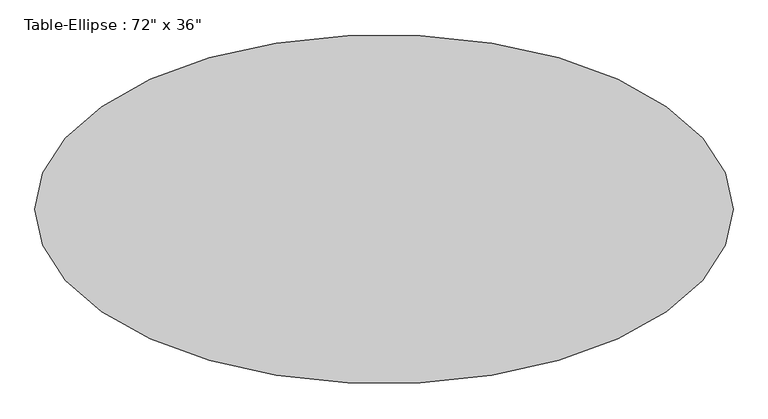
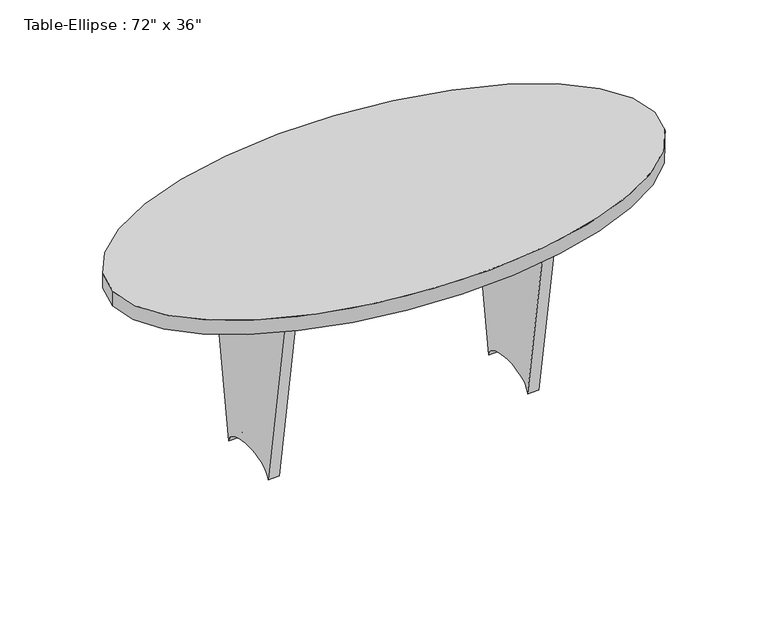
"""IFC4 building model written with IfcOpenShell, lengths in millimetres: furniture geometry."""

from ifc_helpers import new_model, si_unit, point, frame, origin, place, context, project, spatial, ellipse_curve, trimmed, source, transform, mapped, element, save
from ifc_brep_helpers import plane_surface, extruded_surface, advanced_brep


def furniture_027a2ad9(model_context):
    return source(origin(), model_context, "Body", "AdvancedBrep", [
        advanced_brep(
        [(-419.1, 19.05, 711.2), (419.1, 19.05, 711.2), (419.1, 19.05, 474.1333333), (-419.1, 19.05, 474.1333333), (-419.1, -19.05, 711.2), (-419.1, -19.05, 474.1333333), (419.1, -19.05, 474.1333333), (419.1, -19.05, 711.2)],
        [
            (0, 1),
            (1, 2),
            (2, 3, ellipse_curve(frame((0.0, 19.05, 474.1333333), z_axis=(0.0, -1.0, 0.0), x_axis=(1.0, 0.0, 0.0)), 419.1, 101.6)),
            (3, 0),
            (4, 5),
            (5, 6, ellipse_curve(frame((0.0, -19.05, 474.1333333), z_axis=(0.0, 1.0, 0.0), x_axis=(1.0, 0.0, 0.0)), 419.1, 101.6)),
            (6, 7),
            (7, 4),
            (0, 4),
            (7, 1),
            (6, 2),
            (5, 3),
        ],
        [
            plane_surface(frame((-419.1, 19.05, 711.2), z_axis=(0.0, 1.0, 0.0), x_axis=(1.0, 0.0, 0.0))),
            plane_surface(frame((-419.1, -19.05, 711.2), z_axis=(0.0, -1.0, 0.0), x_axis=(-1.0, 0.0, 0.0))),
            plane_surface(frame((-419.1, 19.05, 711.2), z_axis=(0.0, 0.0, 1.0), x_axis=(0.0, -1.0, 0.0))),
            plane_surface(frame((419.1, 19.05, 711.2), z_axis=(1.0, 0.0, 0.0), x_axis=(0.0, -1.0, 0.0))),
            extruded_surface(trimmed(ellipse_curve(frame((0.0, -57.15, 474.1333333), z_axis=(0.0, -1.0, 0.0), x_axis=(1.0, 0.0, 0.0)), 419.1, 101.6), [point((419.1, -57.15, 474.1333333))], [point((-419.1, -57.15, 474.1333333))], True, "CARTESIAN"), (0.0, 38.099999999999994, 0.0), 38.099999999999994),
            plane_surface(frame((-419.1, 19.05, 474.1333333), z_axis=(-1.0, 0.0, 0.0), x_axis=(0.0, -1.0, 0.0))),
        ],
        [
            (0, [[1, 2, 3, 4]]),
            (1, [[5, 6, 7, 8]]),
            (2, [[-1, 9, -8, 10]]),
            (3, [[-2, -10, -7, 11]]),
            (4, [[-3, -11, -6, 12]]),
            (5, [[-4, -12, -5, -9]]),
        ],
    ),
        advanced_brep(
        [(457.2, 228.6, 711.2), (457.2, -228.6, 711.2), (457.2, -114.3, 0.0), (457.2, 114.3, 0.0), (419.1, 228.6, 711.2), (419.1, 114.3, 0.0), (419.1, -114.3, 0.0), (419.1, -228.6, 711.2)],
        [
            (0, 1),
            (1, 2),
            (2, 3, ellipse_curve(frame((457.2, 0.0, 0.0), z_axis=(-1.0, 0.0, 0.0), x_axis=(0.0, 1.0, 0.0)), 114.3, 50.8)),
            (3, 0),
            (4, 5),
            (5, 6, ellipse_curve(frame((419.1, 0.0, 0.0), z_axis=(1.0, 0.0, 0.0), x_axis=(0.0, 1.0, 0.0)), 114.3, 50.8)),
            (6, 7),
            (7, 4),
            (0, 4),
            (7, 1),
            (6, 2),
            (5, 3),
        ],
        [
            plane_surface(frame((457.2, -228.6, 711.2), z_axis=(1.0, 0.0, 0.0), x_axis=(0.0, -1.0, 0.0))),
            plane_surface(frame((419.1, -228.6, 711.2), z_axis=(-1.0, 0.0, 0.0), x_axis=(0.0, 1.0, 0.0))),
            plane_surface(frame((457.2, 228.6, 711.2), z_axis=(0.0, 0.0, 1.0), x_axis=(-1.0, 0.0, 0.0))),
            plane_surface(frame((457.2, -228.6, 711.2), z_axis=(0.0, -0.9873303712766982, -0.158678095383759), x_axis=(-1.0, 0.0, 0.0))),
            extruded_surface(trimmed(ellipse_curve(frame((381.0, 0.0, 0.0), z_axis=(-1.0, 0.0, 0.0), x_axis=(0.0, 1.0, 0.0)), 114.3, 50.8), [point((381.0, -114.3, 0.0))], [point((381.0, 114.3, 0.0))], True, "CARTESIAN"), (38.10000000000002, 0.0, 0.0), 38.10000000000002),
            plane_surface(frame((457.2, 114.3, 0.0), z_axis=(0.0, 0.9873303712767002, -0.15867809538374666), x_axis=(-1.0, 0.0, 0.0))),
        ],
        [
            (0, [[1, 2, 3, 4]]),
            (1, [[5, 6, 7, 8]]),
            (2, [[-1, 9, -8, 10]]),
            (3, [[-2, -10, -7, 11]]),
            (4, [[-3, -11, -6, 12]]),
            (5, [[-4, -12, -5, -9]]),
        ],
    ),
        advanced_brep(
        [(-419.1, 228.6, 711.2), (-419.1, -228.6, 711.2), (-419.1, -114.3, 0.0), (-419.1, 114.3, 0.0), (-457.2, 228.6, 711.2), (-457.2, 114.3, 0.0), (-457.2, -114.3, 0.0), (-457.2, -228.6, 711.2)],
        [
            (0, 1),
            (1, 2),
            (2, 3, ellipse_curve(frame((-419.1, 0.0, 0.0), z_axis=(-1.0, 0.0, 0.0), x_axis=(0.0, 1.0, 0.0)), 114.3, 50.8)),
            (3, 0),
            (4, 5),
            (5, 6, ellipse_curve(frame((-457.2, 0.0, 0.0), z_axis=(1.0, 0.0, 0.0), x_axis=(0.0, 1.0, 0.0)), 114.3, 50.8)),
            (6, 7),
            (7, 4),
            (0, 4),
            (7, 1),
            (6, 2),
            (5, 3),
        ],
        [
            plane_surface(frame((-419.1, -228.6, 711.2), z_axis=(1.0, 0.0, 0.0), x_axis=(0.0, -1.0, 0.0))),
            plane_surface(frame((-457.2, -228.6, 711.2), z_axis=(-1.0, 0.0, 0.0), x_axis=(0.0, 1.0, 0.0))),
            plane_surface(frame((-419.1, 228.6, 711.2), z_axis=(0.0, 0.0, 1.0), x_axis=(-1.0, 0.0, 0.0))),
            plane_surface(frame((-419.1, -228.6, 711.2), z_axis=(0.0, -0.9873303712766983, -0.15867809538375854), x_axis=(-1.0, 0.0, 0.0))),
            extruded_surface(trimmed(ellipse_curve(frame((-495.3, 0.0, 0.0), z_axis=(-1.0, 0.0, 0.0), x_axis=(0.0, 1.0, 0.0)), 114.3, 50.8), [point((-495.3, -114.3, 0.0))], [point((-495.3, 114.3, 0.0))], True, "CARTESIAN"), (38.10000000000002, 0.0, 0.0), 38.10000000000002),
            plane_surface(frame((-419.1, 114.3, 0.0), z_axis=(0.0, 0.9873303712766998, -0.15867809538374977), x_axis=(-1.0, 0.0, 0.0))),
        ],
        [
            (0, [[1, 2, 3, 4]]),
            (1, [[5, 6, 7, 8]]),
            (2, [[-1, 9, -8, 10]]),
            (3, [[-2, -10, -7, 11]]),
            (4, [[-3, -11, -6, 12]]),
            (5, [[-4, -12, -5, -9]]),
        ],
    ),
        advanced_brep(
        [(-914.4, 0.0, 762.0), (914.4, 0.0, 762.0), (-914.4, 0.0, 711.2), (914.4, 0.0, 711.2)],
        [
            (0, 1, ellipse_curve(frame((0.0, 0.0, 762.0), z_axis=(0.0, 0.0, 1.0), x_axis=(1.0, 0.0, 0.0)), 914.4, 457.2)),
            (1, 0, ellipse_curve(frame((0.0, 0.0, 762.0), z_axis=(0.0, 0.0, 1.0), x_axis=(1.0, 0.0, 0.0)), 914.4, 457.2)),
            (2, 3, ellipse_curve(frame((0.0, 0.0, 711.2), z_axis=(0.0, 0.0, -1.0), x_axis=(1.0, 0.0, 0.0)), 914.4, 457.2)),
            (3, 2, ellipse_curve(frame((0.0, 0.0, 711.2), z_axis=(0.0, 0.0, -1.0), x_axis=(1.0, 0.0, 0.0)), 914.4, 457.2)),
            (0, 2),
            (3, 1),
        ],
        [
            plane_surface(frame((914.4, 0.0, 762.0), z_axis=(0.0, 0.0, 1.0), x_axis=(0.0, 1.0, 0.0))),
            plane_surface(frame((914.4, 0.0, 711.2), z_axis=(0.0, 0.0, -1.0), x_axis=(0.0, -1.0, 0.0))),
            extruded_surface(trimmed(ellipse_curve(frame((0.0, 0.0, 660.4), z_axis=(0.0, 0.0, 1.0), x_axis=(1.0, 0.0, 0.0)), 914.4, 457.2), [point((-914.4, 0.0, 660.4))], [point((914.4, 0.0, 660.4))], True, "CARTESIAN"), (0.0, 0.0, 50.80000000000007), 50.80000000000007),
            extruded_surface(trimmed(ellipse_curve(frame((0.0, 0.0, 660.4), z_axis=(0.0, 0.0, 1.0), x_axis=(1.0, 0.0, 0.0)), 914.4, 457.2), [point((914.4, 0.0, 660.4))], [point((-914.4, 0.0, 660.4))], True, "CARTESIAN"), (0.0, 0.0, 50.80000000000007), 50.80000000000007),
        ],
        [
            (0, [[1, 2]]),
            (1, [[3, 4]]),
            (2, [[-1, 5, -4, 6]]),
            (3, [[-2, -6, -3, -5]]),
        ],
    ),
    ])


if __name__ == "__main__":
    model = new_model("IFC4")
    model_context = context("Model", 3, world=origin())
    ifc_project = project(units=[si_unit("LENGTHUNIT", "METRE", prefix="MILLI")], contexts=[model_context])
    site = spatial("IfcSite", under=ifc_project)
    building = spatial("IfcBuilding", under=site)
    placement = place(None, origin())
    furniture_shape = furniture_027a2ad9(model_context)
    element("IfcFurniture", 1, ObjectType="Table-Ellipse : 72\" x 36\"", at=placement, inside=building, context=model_context, shape_type="MappedRepresentation", body=[
        mapped(furniture_shape, transform((0.0, 0.0, 0.0), x_axis=(1.0, 0.0, 0.0), y_axis=(0.0, 1.0, 0.0), z_axis=(0.0, 0.0, 1.0))),
    ])
    save(model, "model.ifc")

# Revit data of these elements
# Type "Table-Ellipse : 72\" x 36\""
#   Assembly Code = "E2020200"
#   Half Width = 1' - 6"
#   Half Length = 3' - 0"
#   Height = 2' - 6"
#   Length = 6' - 0"
#   Width = 3' - 0"
#   Base Material = Birch
#   Top Material = Laminate - Black
#   Default Elevation = 0
# Element 1 (IfcFurniture, "Table-Ellipse : 72\" x 36\"")
#   Materials on its faces: "Birch", "Laminate - Black"
# Materials
#   "Birch": class "Wood", colour RGB 224 178 126, transparency 0, Description = "Betula Alleghaniensis", Cost = 0
#   "Laminate - Black": colour RGB 0 0 0, transparency 0
